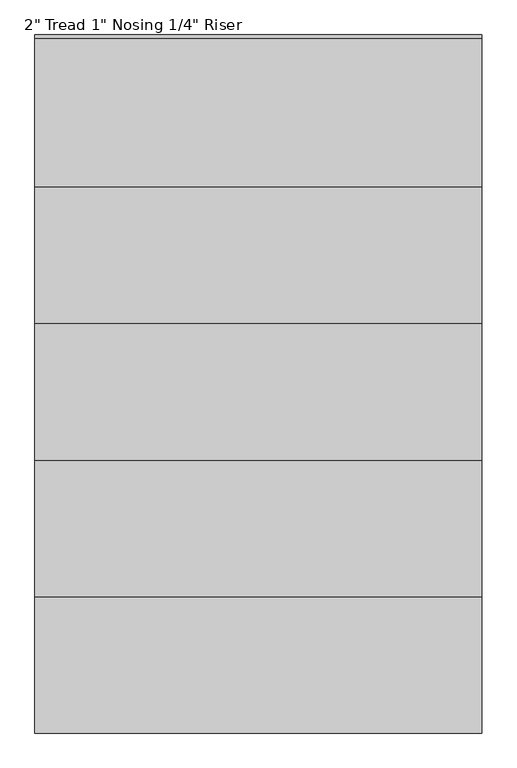
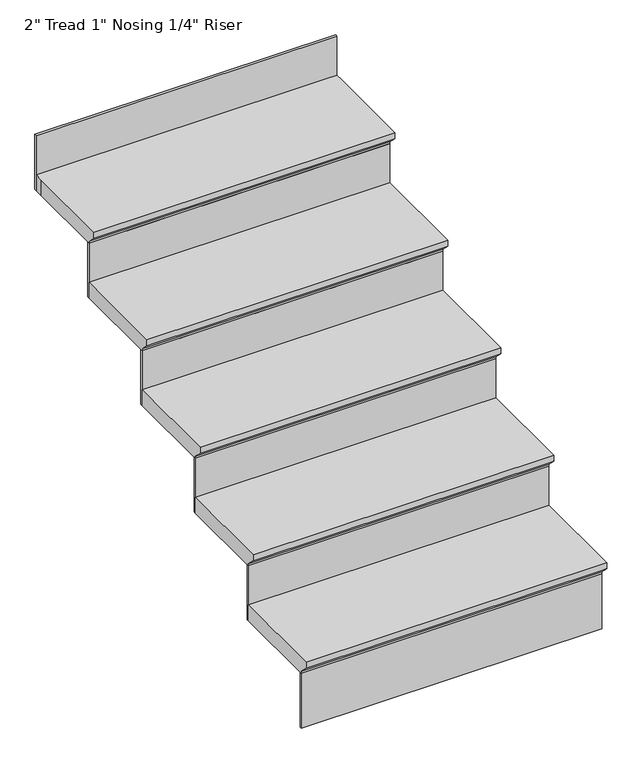
"""IFC4 building model written with IfcOpenShell, lengths in millimetres: stair flight geometry."""

from ifc_helpers import new_model, si_unit, origin, place, context, project, spatial, faceted_brep, source, transform, mapped, element, save


def stair_flight_d68d3b3e(model_context):
    return source(origin(), model_context, "Body", "Brep", [
        faceted_brep([(9871.2423568, -9537.7746824, 4568.9921053), (9871.2423568, -9537.7746824, 4588.0421053), (8956.8423568, -9537.7746824, 4588.0421053), (8956.8423568, -9537.7746824, 4568.9921053), (9871.2423568, -9512.3746824, 4543.5921053), (8956.8423568, -9512.3746824, 4543.5921053), (9871.2423568, -9232.9746824, 4588.0421053), (8956.8423568, -9232.9746824, 4588.0421053), (8956.8423568, -9512.3746824, 4537.2421053), (8956.8423568, -9232.9746824, 4537.2421053), (9871.2423568, -9232.9746824, 4537.2421053), (9871.2423568, -9512.3746824, 4537.2421053)], [[[0, 1, 2, 3]], [[4, 0, 3, 5]], [[2, 1, 6, 7]], [[8, 9, 10, 11]], [[2, 7, 9, 8, 5, 3]], [[8, 11, 4, 5]], [[6, 1, 0, 4, 11, 10]], [[7, 6, 10, 9]]]),
        faceted_brep([(9871.2423568, -9512.3746824, 4537.2421053), (9871.2423568, -9512.3746824, 4360.7789474), (9871.2423568, -9506.0246824, 4360.7789474), (9871.2423568, -9506.0246824, 4537.2421053), (8956.8423568, -9512.3746824, 4537.2421053), (8956.8423568, -9506.0246824, 4537.2421053), (8956.8423568, -9506.0246824, 4360.7789474), (8956.8423568, -9512.3746824, 4360.7789474)], [[[0, 1, 2, 3]], [[4, 5, 6, 7]], [[1, 0, 4, 7]], [[2, 1, 7, 6]], [[3, 2, 6, 5]], [[0, 3, 5, 4]]]),
        faceted_brep([(9871.2423568, -9232.9746824, 4713.7052632), (9871.2423568, -9232.9746824, 4537.2421053), (9871.2423568, -9226.6246824, 4537.2421053), (9871.2423568, -9226.6246824, 4713.7052632), (8956.8423568, -9232.9746824, 4713.7052632), (8956.8423568, -9226.6246824, 4713.7052632), (8956.8423568, -9226.6246824, 4537.2421053), (8956.8423568, -9232.9746824, 4537.2421053)], [[[0, 1, 2, 3]], [[4, 5, 6, 7]], [[1, 0, 4, 7]], [[2, 1, 7, 6]], [[3, 2, 6, 5]], [[0, 3, 5, 4]]]),
        faceted_brep([(8956.8423568, -9258.3746824, 4764.5052632), (9871.2423568, -9258.3746824, 4764.5052632), (9871.2423568, -8953.5746824, 4764.5052632), (8956.8423568, -8953.5746824, 4764.5052632), (8956.8423568, -9232.9746824, 4713.7052632), (8956.8423568, -8953.5746824, 4713.7052632), (9871.2423568, -8953.5746824, 4713.7052632), (9871.2423568, -9232.9746824, 4713.7052632), (8956.8423568, -9232.9746824, 4720.0552632), (8956.8423568, -9258.3746824, 4745.4552632), (9871.2423568, -9232.9746824, 4720.0552632), (9871.2423568, -9258.3746824, 4745.4552632)], [[[0, 1, 2, 3]], [[4, 5, 6, 7]], [[0, 3, 5, 4, 8, 9]], [[4, 7, 10, 8]], [[2, 1, 11, 10, 7, 6]], [[3, 2, 6, 5]], [[11, 1, 0, 9]], [[10, 11, 9, 8]]]),
        faceted_brep([(9871.2423568, -8953.5746824, 4890.1684211), (9871.2423568, -8953.5746824, 4713.7052632), (9871.2423568, -8947.2246824, 4713.7052632), (9871.2423568, -8947.2246824, 4890.1684211), (8956.8423568, -8953.5746824, 4890.1684211), (8956.8423568, -8947.2246824, 4890.1684211), (8956.8423568, -8947.2246824, 4713.7052632), (8956.8423568, -8953.5746824, 4713.7052632)], [[[0, 1, 2, 3]], [[4, 5, 6, 7]], [[1, 0, 4, 7]], [[2, 1, 7, 6]], [[3, 2, 6, 5]], [[0, 3, 5, 4]]]),
        faceted_brep([(8956.8423568, -8978.9746824, 4940.9684211), (9871.2423568, -8978.9746824, 4940.9684211), (9871.2423568, -8674.1746824, 4940.9684211), (8956.8423568, -8674.1746824, 4940.9684211), (8956.8423568, -8953.5746824, 4890.1684211), (8956.8423568, -8674.1746824, 4890.1684211), (9871.2423568, -8674.1746824, 4890.1684211), (9871.2423568, -8953.5746824, 4890.1684211), (8956.8423568, -8953.5746824, 4896.5184211), (8956.8423568, -8978.9746824, 4921.9184211), (9871.2423568, -8953.5746824, 4896.5184211), (9871.2423568, -8978.9746824, 4921.9184211)], [[[0, 1, 2, 3]], [[4, 5, 6, 7]], [[0, 3, 5, 4, 8, 9]], [[4, 7, 10, 8]], [[2, 1, 11, 10, 7, 6]], [[3, 2, 6, 5]], [[11, 1, 0, 9]], [[10, 11, 9, 8]]]),
        faceted_brep([(9871.2423568, -8674.1746824, 5066.6315789), (9871.2423568, -8674.1746824, 4890.1684211), (9871.2423568, -8667.8246824, 4890.1684211), (9871.2423568, -8667.8246824, 5066.6315789), (8956.8423568, -8674.1746824, 5066.6315789), (8956.8423568, -8667.8246824, 5066.6315789), (8956.8423568, -8667.8246824, 4890.1684211), (8956.8423568, -8674.1746824, 4890.1684211)], [[[0, 1, 2, 3]], [[4, 5, 6, 7]], [[1, 0, 4, 7]], [[2, 1, 7, 6]], [[3, 2, 6, 5]], [[0, 3, 5, 4]]]),
        faceted_brep([(8956.8423568, -8699.5746824, 5117.4315789), (9871.2423568, -8699.5746824, 5117.4315789), (9871.2423568, -8394.7746824, 5117.4315789), (8956.8423568, -8394.7746824, 5117.4315789), (8956.8423568, -8674.1746824, 5066.6315789), (8956.8423568, -8394.7746824, 5066.6315789), (9871.2423568, -8394.7746824, 5066.6315789), (9871.2423568, -8674.1746824, 5066.6315789), (8956.8423568, -8674.1746824, 5072.9815789), (8956.8423568, -8699.5746824, 5098.3815789), (9871.2423568, -8674.1746824, 5072.9815789), (9871.2423568, -8699.5746824, 5098.3815789)], [[[0, 1, 2, 3]], [[4, 5, 6, 7]], [[0, 3, 5, 4, 8, 9]], [[4, 7, 10, 8]], [[2, 1, 11, 10, 7, 6]], [[3, 2, 6, 5]], [[11, 1, 0, 9]], [[10, 11, 9, 8]]]),
        faceted_brep([(9871.2423568, -8115.3746824, 5419.5578947), (9871.2423568, -8115.3746824, 5243.0947368), (9871.2423568, -8109.0246824, 5243.0947368), (9871.2423568, -8109.0246824, 5419.5578947), (8956.8423568, -8115.3746824, 5419.5578947), (8956.8423568, -8109.0246824, 5419.5578947), (8956.8423568, -8109.0246824, 5243.0947368), (8956.8423568, -8115.3746824, 5243.0947368)], [[[0, 1, 2, 3]], [[4, 5, 6, 7]], [[1, 0, 4, 7]], [[2, 1, 7, 6]], [[3, 2, 6, 5]], [[0, 3, 5, 4]]]),
        faceted_brep([(9871.2423568, -8394.7746824, 5243.0947368), (9871.2423568, -8394.7746824, 5066.6315789), (9871.2423568, -8388.4246824, 5066.6315789), (9871.2423568, -8388.4246824, 5243.0947368), (8956.8423568, -8394.7746824, 5243.0947368), (8956.8423568, -8388.4246824, 5243.0947368), (8956.8423568, -8388.4246824, 5066.6315789), (8956.8423568, -8394.7746824, 5066.6315789)], [[[0, 1, 2, 3]], [[4, 5, 6, 7]], [[1, 0, 4, 7]], [[2, 1, 7, 6]], [[3, 2, 6, 5]], [[0, 3, 5, 4]]]),
        faceted_brep([(8956.8423568, -8115.3746824, 5293.8947368), (8956.8423568, -8140.7746824, 5293.8947368), (8956.8423568, -8420.1746824, 5293.8947368), (9871.2423568, -8420.1746824, 5293.8947368), (9871.2423568, -8140.7746824, 5293.8947368), (9871.2423568, -8115.3746824, 5293.8947368), (8956.8423568, -8140.7746824, 5243.0947368), (8956.8423568, -8115.3746824, 5243.0947368), (9871.2423568, -8115.3746824, 5243.0947368), (9871.2423568, -8140.7746824, 5243.0947368), (9871.2423568, -8394.7746824, 5243.0947368), (8956.8423568, -8394.7746824, 5243.0947368), (8956.8423568, -8394.7746824, 5249.4447368), (8956.8423568, -8420.1746824, 5274.8447368), (9871.2423568, -8394.7746824, 5249.4447368), (9871.2423568, -8420.1746824, 5274.8447368)], [[[0, 1, 2, 3, 4, 5]], [[6, 7, 8, 9, 10, 11]], [[1, 0, 7, 6]], [[2, 1, 6, 11, 12, 13]], [[11, 10, 14, 12]], [[4, 3, 15, 14, 10, 9]], [[5, 4, 9, 8]], [[0, 5, 8, 7]], [[15, 3, 2, 13]], [[14, 15, 13, 12]]]),
    ])


if __name__ == "__main__":
    model = new_model("IFC4")
    model_context = context("Model", 3, world=origin())
    ifc_project = project(units=[si_unit("LENGTHUNIT", "METRE", prefix="MILLI")], contexts=[model_context])
    site = spatial("IfcSite", under=ifc_project)
    building = spatial("IfcBuilding", under=site)
    placement = place(None, origin())
    stair_flight_shape = stair_flight_d68d3b3e(model_context)
    element("IfcStairFlight", 1, ObjectType="2\" Tread 1\" Nosing 1/4\" Riser", at=placement, inside=building, context=model_context, shape_type="MappedRepresentation", body=[
        mapped(stair_flight_shape, transform((0.0, 0.0, 0.0), x_axis=(1.0, 0.0, 0.0), y_axis=(0.0, 1.0, 0.0), z_axis=(0.0, 0.0, 1.0))),
    ])
    save(model, "model.ifc")

# Revit data of these elements
# Element 1 (IfcStairFlight, "2\" Tread 1\" Nosing 1/4\" Riser")
#   Materials on its faces: "MARBLE STAIRS 6\""
# Materials
#   "MARBLE STAIRS 6\"": class "Generic", colour RGB 120 120 120, transparency 0, Cost = 0
